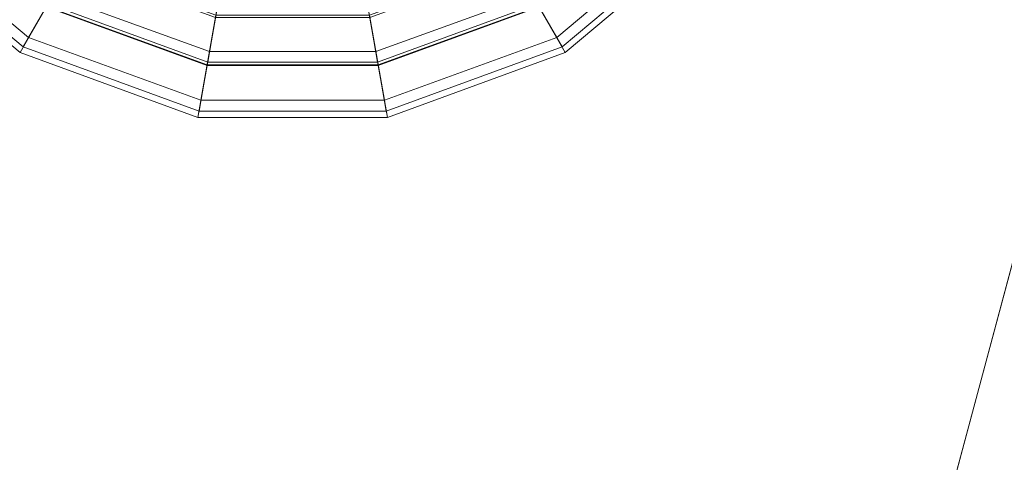
# Model space of a CAD drawing. Units: inches. Extents: x 375 to 1122, y 27 to 1069.
# Tile 139 of 155: x 732.384 to 734.829, y 896.928 to 898.026. Entities that reach past the tile are written whole.
import ezdxf

# ---------------------------------------------------------------- set-up
doc = ezdxf.new("R2010")
doc.units = ezdxf.units.IN
doc.layers.add('A-ANNO-DIMS', color=2, linetype='Continuous', lineweight=18)
doc.layers.add('Furniture', color=30, linetype='Continuous', lineweight=18)
doc.styles.get("Standard").update_dxf_attribs({"font": 'arial.ttf'})
doc.dimstyles.new('ISO-25', dxfattribs={"dimtxt": 12, "dimasz": 2.5, "dimexe": 1.5, "dimexo": 1.5, "dimtad": 1, "dimdec": 1, "dimlunit": 3, "dimtxsty": 'Standard', "dimblk": 'ARCHTICK', "dimcen": 2.5, "dimadec": 0, "dimazin": 0, "dimtfac": 1, "dimtdec": 1, "dimtmove": 0, "dimatfit": 3, "dimfxl": 1.5, "dimfxlon": 1, "dimarcsym": 0})

# ---------------------------------------------------------------- blocks, each defined once
blk = doc.blocks.new('A$C403C54AD')
at = {"linetype": 'ByBlock', "invisible_edges": 5}
for points in [[(1.027872, 1.280047, -0.037345), (1.010941, 1.250721, -0.02811), (1.080205, 1.232162, -0.02811), (1.080205, 1.266024, -0.037345)], [(1.010941, 1.250721, -0.023492), (1.020176, 1.266717, -0.023492), (1.080205, 1.250632, -0.023492), (1.080205, 1.232162, -0.023492)]]:
    blk.add_3dface(points, dxfattribs=at)
at = {"linetype": 'ByBlock'}
blk.add_3dface([(1.010941, 1.250721, -0.02811), (1.010941, 1.250721, -0.023492), (1.080205, 1.232162, -0.023492), (1.080205, 1.232162, -0.02811)], dxfattribs=at)
for points in [[(1.009483, 1.219849, -0.04658), (0.980157, 1.202917, -0.043501), (0.980157, 1.202917, -0.043501), (1.001923, 1.228857, -0.04658)], [(1.00662, 1.218195, 0.116404), (1.009137, 1.219649, 0.10318), (1.001667, 1.228552, 0.10318), (0.999798, 1.226325, 0.116404)], [(1.006655, 1.218216, -0.043349), (1.009483, 1.219849, -0.04658), (1.001923, 1.228857, -0.04658), (0.999824, 1.226356, -0.043349)], [(1.009137, 1.219649, 0.10318), (1.008553, 1.219312, 0.074938), (1.001233, 1.228035, 0.074938), (1.001667, 1.228552, 0.10318)], [(1.008553, 1.219312, 0.074938), (1.003907, 1.216629, 0.056929), (0.997785, 1.223925, 0.056929), (1.001233, 1.228035, 0.074938)], [(1.013505, 1.208798, -0.04658), (0.980157, 1.202917, -0.043501), (0.980157, 1.202917, -0.043501), (1.009483, 1.219849, -0.04658)], [(1.010289, 1.20823, -0.043349), (1.013505, 1.208798, -0.04658), (1.009483, 1.219849, -0.04658), (1.006655, 1.218216, -0.043349)], [(1.012448, 1.208611, 0.074938), (1.007164, 1.20768, 0.056929), (1.003907, 1.216629, 0.056929), (1.008553, 1.219312, 0.074938)], [(1.010249, 1.208223, 0.116404), (1.013112, 1.208728, 0.10318), (1.009137, 1.219649, 0.10318), (1.00662, 1.218195, 0.116404)], [(1.013112, 1.208728, 0.10318), (1.012448, 1.208611, 0.074938), (1.008553, 1.219312, 0.074938), (1.009137, 1.219649, 0.10318)], [(0.994156, 1.205386, -0.040074), (1.010289, 1.20823, -0.043349), (1.006655, 1.218216, -0.043349), (0.992467, 1.210025, -0.040074)], [(1.005329, 1.207356, 0.12581), (1.010249, 1.208223, 0.116404), (1.00662, 1.218195, 0.116404), (1.002293, 1.215697, 0.12581)], [(1.010075, 1.208193, 0.102963), (1.007308, 1.207705, 0.115599), (1.004033, 1.216702, 0.115599), (1.006466, 1.218107, 0.102963)], [(1.009426, 1.208078, 0.075423), (1.010075, 1.208193, 0.102963), (1.006466, 1.218107, 0.102963), (1.005896, 1.217778, 0.075423)], [(1.004396, 1.207191, 0.058276), (1.009426, 1.208078, 0.075423), (1.005896, 1.217778, 0.075423), (1.001473, 1.215224, 0.058276)], [(1.013505, 1.197037, -0.04658), (0.980157, 1.202917, -0.043501), (0.980157, 1.202917, -0.043501), (1.013505, 1.208798, -0.04658)], [(1.010289, 1.197604, -0.043349), (1.013505, 1.197037, -0.04658), (1.013505, 1.208798, -0.04658), (1.010289, 1.20823, -0.043349)], [(0.994156, 1.200449, -0.040074), (1.010289, 1.197604, -0.043349), (1.010289, 1.20823, -0.043349), (0.994156, 1.205386, -0.040074)], [(1.005329, 1.198479, 0.12581), (1.010249, 1.197611, 0.116404), (1.010249, 1.208223, 0.116404), (1.005329, 1.207356, 0.12581)], [(1.012448, 1.197224, 0.074938), (1.007164, 1.198155, 0.056929), (1.007164, 1.20768, 0.056929), (1.012448, 1.208611, 0.074938)], [(1.010075, 1.197642, 0.102963), (1.007308, 1.19813, 0.115599), (1.007308, 1.207705, 0.115599), (1.010075, 1.208193, 0.102963)], [(1.009426, 1.197756, 0.075423), (1.010075, 1.197642, 0.102963), (1.010075, 1.208193, 0.102963), (1.009426, 1.208078, 0.075423)], [(1.010249, 1.197611, 0.116404), (1.013112, 1.197107, 0.10318), (1.013112, 1.208728, 0.10318), (1.010249, 1.208223, 0.116404)], [(1.013112, 1.197107, 0.10318), (1.012448, 1.197224, 0.074938), (1.012448, 1.208611, 0.074938), (1.013112, 1.208728, 0.10318)], [(1.004396, 1.198643, 0.058276), (1.009426, 1.197756, 0.075423), (1.009426, 1.208078, 0.075423), (1.004396, 1.207191, 0.058276)], [(1.009483, 1.185986, -0.04658), (0.980157, 1.202917, -0.043501), (0.980157, 1.202917, -0.043501), (1.013505, 1.197037, -0.04658)], [(1.001923, 1.176977, -0.04658), (0.980157, 1.202917, -0.043501), (0.980157, 1.202917, -0.043501), (1.009483, 1.185986, -0.04658)], [(0.992467, 1.19581, -0.040074), (1.006655, 1.187619, -0.043349), (1.010289, 1.197604, -0.043349), (0.994156, 1.200449, -0.040074)], [(1.001473, 1.190611, 0.058276), (1.005896, 1.188057, 0.075423), (1.009426, 1.197756, 0.075423), (1.004396, 1.198643, 0.058276)], [(1.002293, 1.190138, 0.12581), (1.00662, 1.187639, 0.116404), (1.010249, 1.197611, 0.116404), (1.005329, 1.198479, 0.12581)], [(1.008553, 1.186523, 0.074938), (1.003907, 1.189206, 0.056929), (1.007164, 1.198155, 0.056929), (1.012448, 1.197224, 0.074938)], [(1.006466, 1.187728, 0.102963), (1.004033, 1.189133, 0.115599), (1.007308, 1.19813, 0.115599), (1.010075, 1.197642, 0.102963)], [(1.005896, 1.188057, 0.075423), (1.006466, 1.187728, 0.102963), (1.010075, 1.197642, 0.102963), (1.009426, 1.197756, 0.075423)], [(1.00662, 1.187639, 0.116404), (1.009137, 1.186186, 0.10318), (1.013112, 1.197107, 0.10318), (1.010249, 1.197611, 0.116404)], [(1.006655, 1.187619, -0.043349), (1.009483, 1.185986, -0.04658), (1.013505, 1.197037, -0.04658), (1.010289, 1.197604, -0.043349)], [(1.009137, 1.186186, 0.10318), (1.008553, 1.186523, 0.074938), (1.012448, 1.197224, 0.074938), (1.013112, 1.197107, 0.10318)], [(1.001233, 1.1778, 0.074938), (0.997785, 1.18191, 0.056929), (1.003907, 1.189206, 0.056929), (1.008553, 1.186523, 0.074938)], [(0.999798, 1.17951, 0.116404), (1.001667, 1.177283, 0.10318), (1.009137, 1.186186, 0.10318), (1.00662, 1.187639, 0.116404)], [(0.999824, 1.179479, -0.043349), (1.001923, 1.176977, -0.04658), (1.009483, 1.185986, -0.04658), (1.006655, 1.187619, -0.043349)], [(1.001667, 1.177283, 0.10318), (1.001233, 1.1778, 0.074938), (1.008553, 1.186523, 0.074938), (1.009137, 1.186186, 0.10318)]]:
    blk.add_3dface(points)
blk = doc.blocks.new('_ArchTick')
at = {"color": 0, "linetype": 'ByBlock', "const_width": 0.15}
blk.add_lwpolyline([(-0.5, -0.5), (0.5, 0.5)], dxfattribs=at)
blk = doc.blocks.new('*D88')
at = {"layer": 'A-ANNO-DIMS', "color": 0, "lineweight": -2, "transparency": 16777216}
for p, q in [((731.0073, 1052.5277), (731.0073, 1055.5277)), ((854.0073, 1052.5277), (854.0073, 1055.5277)), ((731.0073, 1054.0277), (854.0073, 1054.0277))]:
    blk.add_line(p, q, dxfattribs=at)
at = {"layer": 'Defpoints', "color": 0, "transparency": 16777216}
for p in [(854.0073, 1054.0277), (731.0073, 502.5277), (854.0073, 502.5277)]:
    blk.add_point(p, dxfattribs=at)
at = {"layer": 'A-ANNO-DIMS', "color": 0, "lineweight": -2, "transparency": 16777216, "xscale": 2.5, "yscale": 2.5, "zscale": 2.5, "rotation": 180}
blk.add_blockref('_ArchTick', (731.0073, 1054.0277), dxfattribs=at)
at = {"layer": 'A-ANNO-DIMS', "color": 0, "lineweight": -2, "transparency": 16777216, "xscale": 2.5, "yscale": 2.5, "zscale": 2.5}
blk.add_blockref('_ArchTick', (854.0073, 1054.0277), dxfattribs=at)
at = {"layer": 'A-ANNO-DIMS', "color": 0, "transparency": 16777216, "insert": (792.5073, 1060.7837), "char_height": 12, "attachment_point": 5}
blk.add_mtext('10\'-3"', dxfattribs=at)
blk = doc.blocks.new('*D91')
at = {"layer": 'A-ANNO-DIMS', "color": 0, "lineweight": -2, "transparency": 16777216}
for p, q in [((728.0073, 1052.5277), (728.0073, 1055.5277)), ((788.0073, 1052.5277), (788.0073, 1055.5277)), ((728.0073, 1054.0277), (788.0073, 1054.0277))]:
    blk.add_line(p, q, dxfattribs=at)
at = {"layer": 'Defpoints', "color": 0, "transparency": 16777216}
for p in [(788.0073, 1054.0277), (728.0073, 774.0277), (788.0073, 774.0277)]:
    blk.add_point(p, dxfattribs=at)
at = {"layer": 'A-ANNO-DIMS', "color": 0, "lineweight": -2, "transparency": 16777216, "xscale": 2.5, "yscale": 2.5, "zscale": 2.5, "rotation": 180}
blk.add_blockref('_ArchTick', (728.0073, 1054.0277), dxfattribs=at)
at = {"layer": 'A-ANNO-DIMS', "color": 0, "lineweight": -2, "transparency": 16777216, "xscale": 2.5, "yscale": 2.5, "zscale": 2.5}
blk.add_blockref('_ArchTick', (788.0073, 1054.0277), dxfattribs=at)
at = {"layer": 'A-ANNO-DIMS', "color": 0, "transparency": 16777216, "insert": (758.0073, 1060.7796), "char_height": 12, "attachment_point": 5}
blk.add_mtext('5\'-0"', dxfattribs=at)

msp = doc.modelspace()

# ---------------------------------------------------------------- block references
at = {"layer": 'Furniture', "xscale": 39.9918517141215, "yscale": 39.9918517141215, "zscale": 39.9918517141215, "rotation": 270}
msp.add_blockref('A$C403C54AD', (684.9549, 938.3156, 0.024), dxfattribs=at)

# ---------------------------------------------------------------- dimensions: what is measured, and where the dimension line sits
at = {"layer": 'A-ANNO-DIMS'}
for base, p1, p2, picture, middle in [((788.0073, 1054.0277), (728.0073, 774.0277), (788.0073, 774.0277), '*D91', (758.0073, 1060.7796)), ((854.0073, 1054.0277), (731.0073, 502.5277), (854.0073, 502.5277), '*D88', (792.5073, 1060.7837))]:
    dim = msp.add_linear_dim(base=base, p1=p1, p2=p2, dimstyle='ISO-25', override={"dimdec": 1, "dimlfac": 1, "dimrnd": 0, "dimzin": 1, "dimdsep": 46, "dimlunit": 4, "dimfrac": 2}, dxfattribs=at)
    dim.commit()
    dim.dimension.update_dxf_attribs({"geometry": picture, "text_midpoint": middle})

doc.saveas('drawing.dxf')
